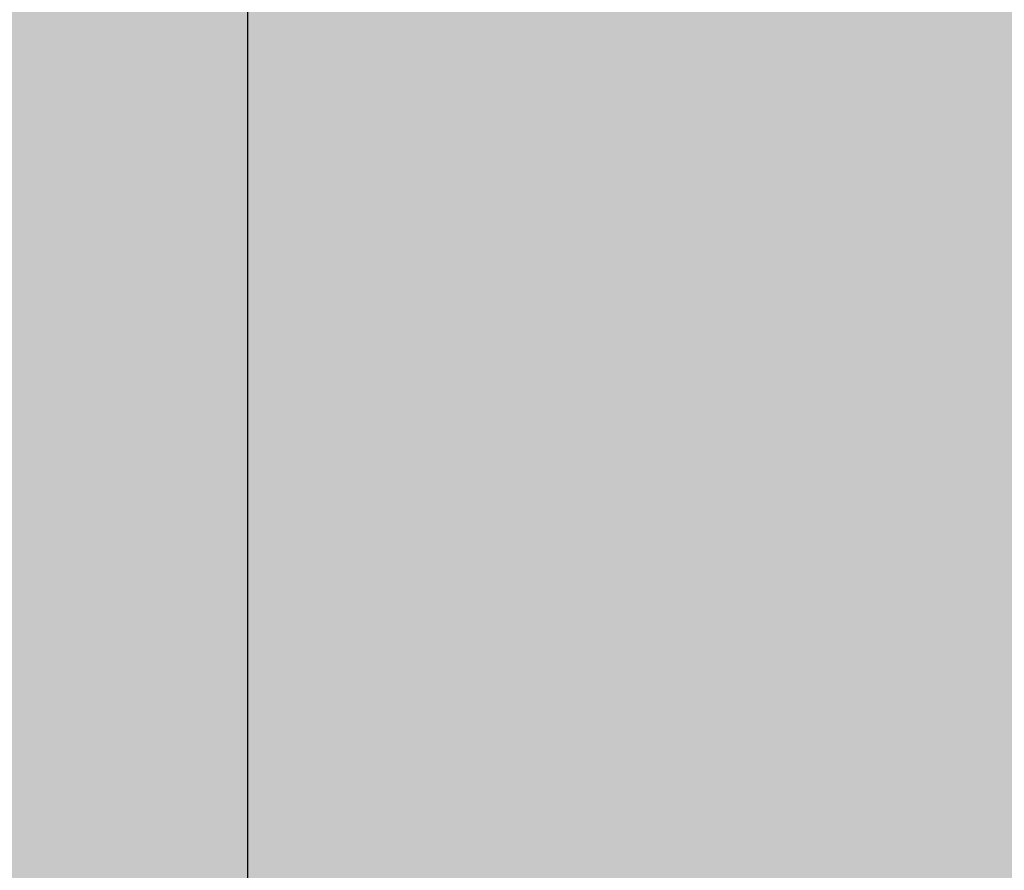
# Model space of a CAD drawing. Units: millimetres. Extents: x -22994 to 29398, y -19990 to 20176.
# Tile 64 of 135: x 225.2725 to 225.8137, y 83.796 to 84.2638. Entities that reach past the tile are written whole.
import ezdxf

# ---------------------------------------------------------------- set-up
doc = ezdxf.new("R2010")
doc.units = ezdxf.units.MM
doc.header["$MEASUREMENT"] = 0
doc.layers.add('M-EQPM', color=7, linetype='Continuous', lineweight=25)
doc.layers.add('M-EQPM-PATT', color=7, linetype='Continuous', lineweight=18)

msp = doc.modelspace()

# ---------------------------------------------------------------- hatches: boundary and pattern name
at = {"layer": 'M-EQPM-PATT'}
h = msp.add_hatch(color=256, dxfattribs=at)
h.set_gradient(color1=(205, 32, 39), color2=(205, 32, 39), tint=1)
h.paths.add_polyline_path([(116.26467, 150.36616), (116.26467, 170.36616), (116.26467, 176.36616), (110.26467, 176.36616), (110.26467, 152.02763), (95.83267, 127.96702), (95.83267, 16.60628), (201.69668, 16.60628), (201.69668, 127.96702), (187.26467, 152.02763), (187.26467, 176.36616), (181.26467, 176.36616), (181.26467, 170.36616), (181.26467, 150.36616), (195.69668, 126.30555), (195.69668, 22.60628), (101.83267, 22.60628), (101.83267, 126.30555)])
h.paths.add_polyline_path([(185.22083, 88.63474), (101.83267, 88.63474), (101.83267, 87.63474), (182.80661, 87.63474), (178.73126, 83.55939), (195.69668, 83.55939), (195.69668, 84.55939), (181.14547, 84.55939)], flags=17)
h.paths.add_polyline_path([(95.83267, 88.63474), (60.97786, 88.63474, -0.022855), (61.71782, 87.63474), (95.83267, 87.63474)])
h.paths.add_polyline_path([(215.62123, 86.51891), (215.62123, 80.59986), (220.50954, 83.55939)])
h.paths.add_polyline_path([(215.62123, 84.55939), (201.69668, 84.55939), (201.69668, 83.55939), (215.62123, 83.55939)])
h.paths.add_polyline_path([(225.39784, 86.51891), (220.50954, 83.55939), (225.39784, 80.59986)])
h.paths.add_polyline_path([(231.62561, 84.55939), (225.39784, 84.55939), (225.39784, 83.55939), (231.62561, 83.55939)])

# ---------------------------------------------------------------- linework, layer by layer
at = {"layer": 'M-EQPM'}
msp.add_lwpolyline([(225.39784, 86.51891), (215.62123, 80.59986), (215.62123, 86.51891), (225.39784, 80.59986)], close=True, dxfattribs=at)

doc.saveas('drawing.dxf')
